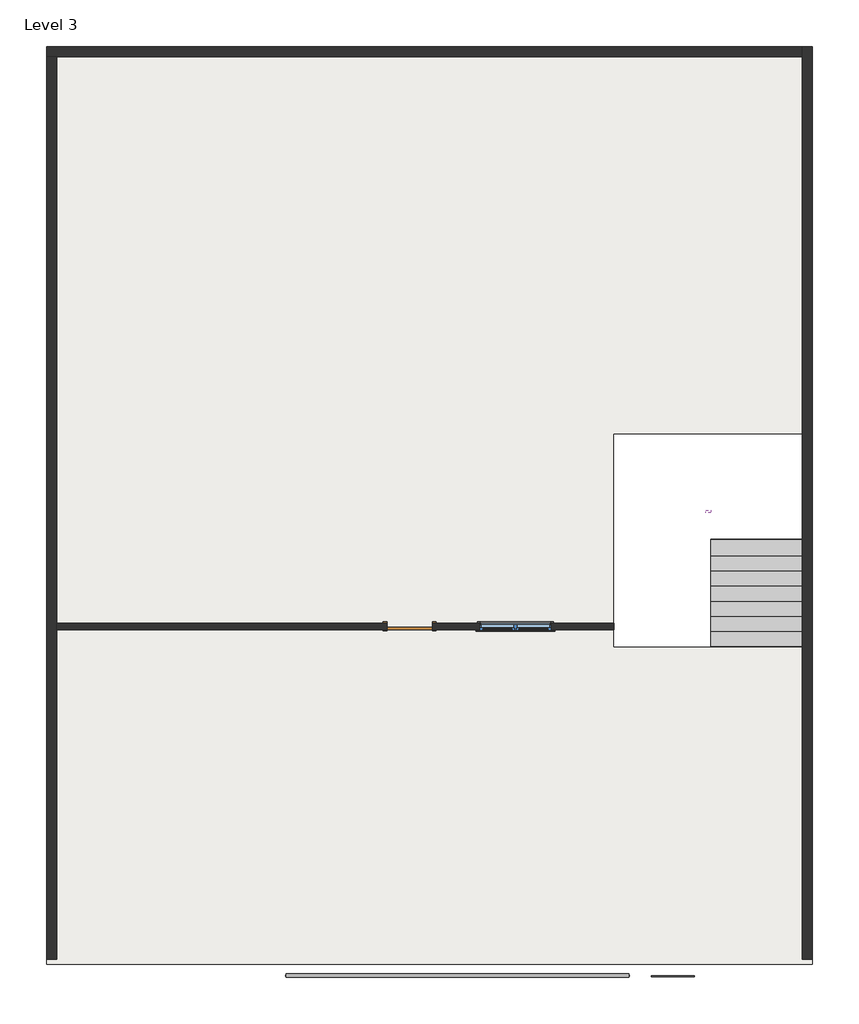
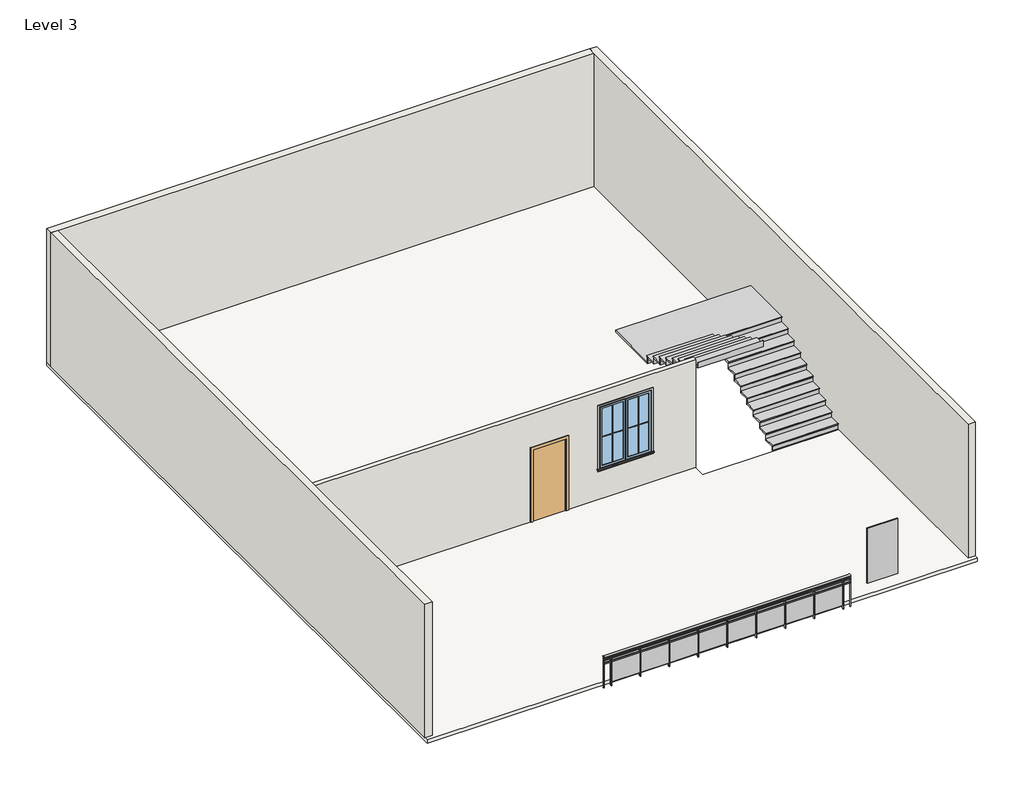
# One storey: 4 proxies, 4 walls, 1 door, 1 member, 1 plate, 1 railing, 1 slab, 1 stair flight, 1 window.
"""IFC4 building model written with IfcOpenShell, lengths in millimetres."""

from ifc_helpers import new_model, si_unit, point, frame, origin, place, context, project, spatial, polyline, ellipse_curve, trimmed, outline, extrude, faceted_brep, transform, mapped, element, save
from ifc_brep_helpers import plane_surface, extruded_surface, advanced_brep
from components import muntin_pattern_2x2_muntin_pattern_2x2_bff912c5, muntin_pattern_2x2_muntin_pattern_2x2_c2194282, trim_window_exterior_flat_with_sill_e04b3088, trim_window_interior_flat_picture_frame_2a7685fe, door_a1797ceb, system_panel_glazed_1c5a620b, stair_flight_059c6031, window_51a0d18f

model = new_model("IFC4")

# Units and contexts
model_context = context("Model", 3, world=origin())
ifc_project = project(units=[si_unit("LENGTHUNIT", "METRE", prefix="MILLI")], contexts=[model_context])

# Site, building, storey
site = spatial("IfcSite", under=ifc_project)
building = spatial("IfcBuilding", under=site)
storey = spatial("IfcBuildingStorey", under=building, Name="Level 3", Elevation=3962.4)

# Proxies
placement = place(None, origin())
muntin_pattern_2x2_muntin_pattern_2x2_shape = muntin_pattern_2x2_muntin_pattern_2x2_bff912c5(model_context)
element("IfcBuildingElementProxy", 1, Name="Muntin Pattern_2x2 : Muntin Pattern_2x2", ObjectType="Muntin Pattern_2x2 : Muntin Pattern_2x2", at=placement, inside=storey, context=model_context, shape_type="MappedRepresentation", body=[
    mapped(muntin_pattern_2x2_muntin_pattern_2x2_shape, transform((2360.2518946, -8297.1080955, 4946.65), x_axis=(-1.0, 0.0, 0.0), y_axis=(0.0, -1.0, 0.0), z_axis=(0.0, 0.0, 1.0))),
])
muntin_pattern_2x2_muntin_pattern_2x2_2_shape = muntin_pattern_2x2_muntin_pattern_2x2_c2194282(model_context)
element("IfcBuildingElementProxy", 2, Name="Muntin Pattern_2x2 : Muntin Pattern_2x2", ObjectType="Muntin Pattern_2x2 : Muntin Pattern_2x2", at=placement, inside=storey, context=model_context, shape_type="MappedRepresentation", body=[
    mapped(muntin_pattern_2x2_muntin_pattern_2x2_2_shape, transform((1639.5268946, -8297.1080955, 4946.65), x_axis=(1.0, 0.0, 0.0), y_axis=(0.0, 1.0, 0.0), z_axis=(0.0, 0.0, 1.0))),
])
trim_window_exterior_flat_with_sill_shape = trim_window_exterior_flat_with_sill_e04b3088(model_context)
element("IfcBuildingElementProxy", 3, Name="Trim-Window-Exterior-Flat : with Sill", ObjectType="Trim-Window-Exterior-Flat : with Sill", at=placement, inside=storey, context=model_context, shape_type="MappedRepresentation", body=[
    mapped(trim_window_exterior_flat_with_sill_shape, transform((1999.8893946, -8306.6330955, 6705.6), x_axis=(1.0, 0.0, 0.0), y_axis=(0.0, 0.0, 1.0), z_axis=(0.0, -1.0, 0.0))),
])
trim_window_interior_flat_picture_frame_shape = trim_window_interior_flat_picture_frame_2a7685fe(model_context)
element("IfcBuildingElementProxy", 4, Name="Trim-Window-Interior-Flat : Picture Frame", ObjectType="Trim-Window-Interior-Flat : Picture Frame", at=placement, inside=storey, context=model_context, shape_type="MappedRepresentation", body=[
    mapped(trim_window_interior_flat_picture_frame_shape, transform((1999.8893946, -8179.6330955, 6705.6), x_axis=(-1.0, 0.0, 0.0), y_axis=(0.0, 0.0, 1.0), z_axis=(0.0, 1.0, 0.0))),
])

# Door
door_shape = door_a1797ceb(model_context)
element("IfcDoor", 5, ObjectType="Single-Flush : 36\" x 84\"", at=placement, inside=storey, context=model_context, shape_type="MappedRepresentation", body=[
    mapped(door_shape, transform((-133.7106054, -8243.1330955, 3962.4), x_axis=(-1.0, 0.0, 0.0), y_axis=(0.0, -1.0, 0.0), z_axis=(0.0, 0.0, 1.0))),
])

# Member
element("IfcMember", 6, ObjectType="Stringer - 2\" Width", at=placement, inside=storey, context=model_context, shape_type="SweptSolid", body=[
    extrude(outline(polyline([(5940.6255016, -5904.9976656), (5940.6255016, -5955.7976656), (5839.0255016, -5955.7976656), (5839.0255016, -5904.9976656), (5940.6255016, -5904.9976656)])), frame((0.0, 0.0, 5418.2210526), z_axis=(0.0, 0.0, 1.0), x_axis=(1.0, 0.0, 0.0)), (0.0, 0.0, 1.0), 304.8),
])

# Plate
system_panel_glazed_shape = system_panel_glazed_1c5a620b(model_context)
element("IfcPlate", 7, ObjectType="System Panel : Glazed", at=placement, inside=storey, context=model_context, shape_type="MappedRepresentation", body=[
    mapped(system_panel_glazed_shape, transform((5174.2954883, -15325.4077095, 4495.8), x_axis=(1.0, 0.0, 0.0), y_axis=(0.0, 1.0, 0.0), z_axis=(0.0, 0.0, 1.0))),
])

# Railing
element("IfcRailing", 8, ObjectType="Glass Panel - Bottom Fill", at=placement, inside=storey, context=model_context, shape_type="SolidModel", body=[
    advanced_brep(
    [(-2628.7186876, -15240.8330955, 4876.8), (-2628.7186876, -15317.0330955, 4876.8), (4285.8893946, -15240.8330955, 4876.8), (4285.8893946, -15317.0330955, 4876.8)],
    [
        (0, 1, ellipse_curve(frame((-2628.7186876, -15278.9330955, 4876.8), z_axis=(-1.0, 0.0, 0.0), x_axis=(0.0, -1.0, 0.0)), 38.1, 28.575)),
        (1, 0, ellipse_curve(frame((-2628.7186876, -15278.9330955, 4876.8), z_axis=(-1.0, 0.0, 0.0), x_axis=(0.0, -1.0, 0.0)), 38.1, 28.575)),
        (2, 3, ellipse_curve(frame((4285.8893946, -15278.9330955, 4876.8), z_axis=(1.0, 0.0, 0.0), x_axis=(0.0, -1.0, 0.0)), 38.1, 28.575)),
        (3, 2, ellipse_curve(frame((4285.8893946, -15278.9330955, 4876.8), z_axis=(1.0, 0.0, 0.0), x_axis=(0.0, -1.0, 0.0)), 38.1, 28.575)),
        (0, 2),
        (3, 1),
    ],
    [
        plane_surface(frame((-2628.7186876, -15278.9330955, 4876.8), z_axis=(-1.0, 0.0, 0.0), x_axis=(0.0, 1.0, 0.0))),
        plane_surface(frame((4285.8893946, -15278.9330955, 4876.8), z_axis=(1.0, 0.0, 0.0), x_axis=(0.0, 1.0, 0.0))),
        extruded_surface(trimmed(ellipse_curve(frame((4285.8893946, -15278.9330955, 4876.8), z_axis=(-1.0, 0.0, 0.0), x_axis=(0.0, -1.0, 0.0)), 38.1, 28.575), [point((4285.8893946, -15240.8330955, 4876.8))], [point((4285.8893946, -15317.0330955, 4876.8))], True, "CARTESIAN"), (-6914.6080822, 0.0, 0.0), 6914.6080822),
        extruded_surface(trimmed(ellipse_curve(frame((4285.8893946, -15278.9330955, 4876.8), z_axis=(-1.0, 0.0, 0.0), x_axis=(0.0, -1.0, 0.0)), 38.1, 28.575), [point((4285.8893946, -15317.0330955, 4876.8))], [point((4285.8893946, -15240.8330955, 4876.8))], True, "CARTESIAN"), (-6914.6080822, 0.0, 0.0), 6914.6080822),
    ],
    [
        (0, [[1, 2]]),
        (1, [[3, 4]]),
        (2, [[-1, 5, -4, 6]]),
        (3, [[-2, -6, -3, -5]]),
    ],
),
    extrude(outline(polyline([(-2628.7186876, -15291.6330955), (-2628.7186876, -15266.2330955), (4285.8893946, -15266.2330955), (4285.8893946, -15291.6330955), (-2628.7186876, -15291.6330955)])), frame((0.0, 0.0, 4762.5), z_axis=(0.0, 0.0, 1.0), x_axis=(1.0, 0.0, 0.0)), (0.0, 0.0, 1.0), 25.4),
    extrude(outline(polyline([(-2628.7186876, -15291.6330955), (-2628.7186876, -15266.2330955), (4285.8893946, -15266.2330955), (4285.8893946, -15291.6330955), (-2628.7186876, -15291.6330955)])), frame((0.0, 0.0, 4660.9), z_axis=(0.0, 0.0, 1.0), x_axis=(1.0, 0.0, 0.0)), (0.0, 0.0, 1.0), 25.4),
    extrude(outline(polyline([(4073.4353535, -15304.3330955), (4073.4353535, -15253.5330955), (4086.1353535, -15253.5330955), (4086.1353535, -15304.3330955), (4073.4353535, -15304.3330955)])), frame((0.0, 0.0, 3962.4), z_axis=(0.0, 0.0, 1.0), x_axis=(1.0, 0.0, 0.0)), (0.0, 0.0, 1.0), 885.6788223),
    extrude(outline(polyline([(3266.9853535, -15272.3979385), (4079.7853535, -15272.3979385), (4079.7853535, -15278.7479385), (3266.9853535, -15278.7479385), (3266.9853535, -15272.3979385)])), frame((0.0, 0.0, 4064.0), z_axis=(0.0, 0.0, 1.0), x_axis=(1.0, 0.0, 0.0)), (0.0, 0.0, 1.0), 596.9),
    extrude(outline(polyline([(3260.6353535, -15304.3330955), (3260.6353535, -15253.5330955), (3273.3353535, -15253.5330955), (3273.3353535, -15304.3330955), (3260.6353535, -15304.3330955)])), frame((0.0, 0.0, 3962.4), z_axis=(0.0, 0.0, 1.0), x_axis=(1.0, 0.0, 0.0)), (0.0, 0.0, 1.0), 885.6788223),
    extrude(outline(polyline([(2454.1853535, -15272.3979385), (3266.9853535, -15272.3979385), (3266.9853535, -15278.7479385), (2454.1853535, -15278.7479385), (2454.1853535, -15272.3979385)])), frame((0.0, 0.0, 4064.0), z_axis=(0.0, 0.0, 1.0), x_axis=(1.0, 0.0, 0.0)), (0.0, 0.0, 1.0), 596.9),
    extrude(outline(polyline([(2447.8353535, -15304.3330955), (2447.8353535, -15253.5330955), (2460.5353535, -15253.5330955), (2460.5353535, -15304.3330955), (2447.8353535, -15304.3330955)])), frame((0.0, 0.0, 3962.4), z_axis=(0.0, 0.0, 1.0), x_axis=(1.0, 0.0, 0.0)), (0.0, 0.0, 1.0), 885.6788223),
    extrude(outline(polyline([(1641.3853535, -15272.3979385), (2454.1853535, -15272.3979385), (2454.1853535, -15278.7479385), (1641.3853535, -15278.7479385), (1641.3853535, -15272.3979385)])), frame((0.0, 0.0, 4064.0), z_axis=(0.0, 0.0, 1.0), x_axis=(1.0, 0.0, 0.0)), (0.0, 0.0, 1.0), 596.9),
    extrude(outline(polyline([(1635.0353535, -15304.3330955), (1635.0353535, -15253.5330955), (1647.7353535, -15253.5330955), (1647.7353535, -15304.3330955), (1635.0353535, -15304.3330955)])), frame((0.0, 0.0, 3962.4), z_axis=(0.0, 0.0, 1.0), x_axis=(1.0, 0.0, 0.0)), (0.0, 0.0, 1.0), 885.6788223),
    extrude(outline(polyline([(828.5853535, -15272.3979385), (1641.3853535, -15272.3979385), (1641.3853535, -15278.7479385), (828.5853535, -15278.7479385), (828.5853535, -15272.3979385)])), frame((0.0, 0.0, 4064.0), z_axis=(0.0, 0.0, 1.0), x_axis=(1.0, 0.0, 0.0)), (0.0, 0.0, 1.0), 596.9),
    extrude(outline(polyline([(822.2353535, -15304.3330955), (822.2353535, -15253.5330955), (834.9353535, -15253.5330955), (834.9353535, -15304.3330955), (822.2353535, -15304.3330955)])), frame((0.0, 0.0, 3962.4), z_axis=(0.0, 0.0, 1.0), x_axis=(1.0, 0.0, 0.0)), (0.0, 0.0, 1.0), 885.6788223),
    extrude(outline(polyline([(15.7853535, -15272.3979385), (828.5853535, -15272.3979385), (828.5853535, -15278.7479385), (15.7853535, -15278.7479385), (15.7853535, -15272.3979385)])), frame((0.0, 0.0, 4064.0), z_axis=(0.0, 0.0, 1.0), x_axis=(1.0, 0.0, 0.0)), (0.0, 0.0, 1.0), 596.9),
    extrude(outline(polyline([(9.4353535, -15304.3330955), (9.4353535, -15253.5330955), (22.1353535, -15253.5330955), (22.1353535, -15304.3330955), (9.4353535, -15304.3330955)])), frame((0.0, 0.0, 3962.4), z_axis=(0.0, 0.0, 1.0), x_axis=(1.0, 0.0, 0.0)), (0.0, 0.0, 1.0), 885.6788223),
    extrude(outline(polyline([(-797.0146465, -15272.3979385), (15.7853535, -15272.3979385), (15.7853535, -15278.7479385), (-797.0146465, -15278.7479385), (-797.0146465, -15272.3979385)])), frame((0.0, 0.0, 4064.0), z_axis=(0.0, 0.0, 1.0), x_axis=(1.0, 0.0, 0.0)), (0.0, 0.0, 1.0), 596.9),
    extrude(outline(polyline([(-803.3646465, -15304.3330955), (-803.3646465, -15253.5330955), (-790.6646465, -15253.5330955), (-790.6646465, -15304.3330955), (-803.3646465, -15304.3330955)])), frame((0.0, 0.0, 3962.4), z_axis=(0.0, 0.0, 1.0), x_axis=(1.0, 0.0, 0.0)), (0.0, 0.0, 1.0), 885.6788223),
    extrude(outline(polyline([(-1609.8146465, -15272.3979385), (-797.0146465, -15272.3979385), (-797.0146465, -15278.7479385), (-1609.8146465, -15278.7479385), (-1609.8146465, -15272.3979385)])), frame((0.0, 0.0, 4064.0), z_axis=(0.0, 0.0, 1.0), x_axis=(1.0, 0.0, 0.0)), (0.0, 0.0, 1.0), 596.9),
    extrude(outline(polyline([(-1616.1646465, -15304.3330955), (-1616.1646465, -15253.5330955), (-1603.4646465, -15253.5330955), (-1603.4646465, -15304.3330955), (-1616.1646465, -15304.3330955)])), frame((0.0, 0.0, 3962.4), z_axis=(0.0, 0.0, 1.0), x_axis=(1.0, 0.0, 0.0)), (0.0, 0.0, 1.0), 885.6788223),
    extrude(outline(polyline([(-2422.6146465, -15272.3979385), (-1609.8146465, -15272.3979385), (-1609.8146465, -15278.7479385), (-2422.6146465, -15278.7479385), (-2422.6146465, -15272.3979385)])), frame((0.0, 0.0, 4064.0), z_axis=(0.0, 0.0, 1.0), x_axis=(1.0, 0.0, 0.0)), (0.0, 0.0, 1.0), 596.9),
    extrude(outline(polyline([(-2428.9646465, -15304.3330955), (-2428.9646465, -15253.5330955), (-2416.2646465, -15253.5330955), (-2416.2646465, -15304.3330955), (-2428.9646465, -15304.3330955)])), frame((0.0, 0.0, 3962.4), z_axis=(0.0, 0.0, 1.0), x_axis=(1.0, 0.0, 0.0)), (0.0, 0.0, 1.0), 885.6788223),
    extrude(outline(polyline([(4273.1893946, -15288.4580955), (4273.1893946, -15269.4080955), (4292.2393946, -15269.4080955), (4292.2393946, -15288.4580955), (4273.1893946, -15288.4580955)])), frame((0.0, 0.0, 3962.4), z_axis=(0.0, 0.0, 1.0), x_axis=(1.0, 0.0, 0.0)), (0.0, 0.0, 1.0), 885.6788223),
    extrude(outline(polyline([(-2635.0686876, -15288.4580955), (-2635.0686876, -15269.4080955), (-2616.0186876, -15269.4080955), (-2616.0186876, -15288.4580955), (-2635.0686876, -15288.4580955)])), frame((0.0, 0.0, 3962.4), z_axis=(0.0, 0.0, 1.0), x_axis=(1.0, 0.0, 0.0)), (0.0, 0.0, 1.0), 885.6788223),
])

# Slab
element("IfcSlab", 9, ObjectType="Generic - 4\"", at=placement, inside=storey, context=model_context, shape_type="SweptSolid", body=[
    extrude(outline(polyline([(-7454.7186876, -15050.3330955), (-7454.7186876, 3440.8669045), (7988.4813124, 3440.8669045), (7988.4813124, -15050.3330955), (-7454.7186876, -15050.3330955)]), holes=[polyline([(7797.9813124, -4367.7173694), (3981.0893946, -4367.7173694), (3981.0893946, -8648.1976656), (7797.9813124, -8648.1976656), (7797.9813124, -4367.7173694)])]), frame((0.0, 0.0, 3860.8), z_axis=(0.0, 0.0, 1.0), x_axis=(1.0, 0.0, 0.0)), (0.0, 0.0, 1.0), 101.6),
])

# Stair flight
stair_flight_shape = stair_flight_059c6031(model_context)
element("IfcStairFlight", 10, ObjectType="2\" Tread 1\" Nosing 1/4\" Riser", at=placement, inside=storey, context=model_context, shape_type="MappedRepresentation", body=[
    mapped(stair_flight_shape, transform((0.0, 0.0, 0.0), x_axis=(1.0, 0.0, 0.0), y_axis=(0.0, 1.0, 0.0), z_axis=(0.0, 0.0, 1.0))),
])

# Walls
element("IfcWall", 11, ObjectType="Generic - 5\"", at=placement, inside=storey, context=model_context, shape_type="SweptSolid", body=[
    extrude(outline(polyline([(3962.4, -7251.5186876), (3962.4, -590.9106054), (6096.0, -590.9106054), (6096.0, 323.4893946), (3962.4, 323.4893946), (3962.4, 3981.0893946), (7162.8, 3981.0893946), (7162.8, -7251.5186876), (3962.4, -7251.5186876)]), holes=[polyline([(6705.6, 1275.9893946), (6705.6, 2723.7893946), (4876.8, 2723.7893946), (4876.8, 1275.9893946), (6705.6, 1275.9893946)])]), frame((0.0, -8306.6330955, 0.0), z_axis=(0.0, 1.0, 0.0), x_axis=(0.0, 0.0, 1.0)), (0.0, 0.0, 1.0), 127.0),
])
element("IfcWall", 12, ObjectType="Generic - 8\"", at=placement, inside=storey, context=model_context, shape_type="Brep", body=[
    faceted_brep([(7988.4813124, -14948.7330955, 3962.4), (7988.4813124, 3440.8669045, 3962.4), (7988.4813124, 3440.8669045, 7924.8), (7988.4813124, -14948.7330955, 7924.8), (7785.2813124, -14948.7330955, 3962.4), (7785.2813124, -14948.7330955, 7924.8), (7785.2813124, 3237.6669045, 7924.8), (7785.2813124, 3440.8669045, 7924.8), (7785.2813124, 3440.8669045, 3962.4), (7785.2813124, 3237.6669045, 3962.4)], [[[0, 1, 2, 3]], [[4, 5, 6, 7, 8, 9]], [[1, 0, 4, 9, 8]], [[3, 2, 7, 6, 5]], [[0, 3, 5, 4]], [[2, 1, 8, 7]]]),
])
element("IfcWall", 13, ObjectType="Generic - 8\"", at=placement, inside=storey, context=model_context, shape_type="Brep", body=[
    faceted_brep([(7785.2813124, 3440.8669045, 3962.4), (-7454.7186876, 3440.8669045, 3962.4), (-7454.7186876, 3440.8669045, 7924.8), (7785.2813124, 3440.8669045, 7924.8), (7785.2813124, 3237.6669045, 3962.4), (7785.2813124, 3237.6669045, 7924.8), (-7251.5186876, 3237.6669045, 7924.8), (-7454.7186876, 3237.6669045, 7924.8), (-7454.7186876, 3237.6669045, 3962.4), (-7251.5186876, 3237.6669045, 3962.4)], [[[0, 1, 2, 3]], [[4, 5, 6, 7, 8, 9]], [[1, 0, 4, 9, 8]], [[3, 2, 7, 6, 5]], [[0, 3, 5, 4]], [[2, 1, 8, 7]]]),
])
element("IfcWall", 14, ObjectType="Generic - 8\"", at=placement, inside=storey, context=model_context, shape_type="Brep", body=[
    faceted_brep([(-7454.7186876, 3237.6669045, 3962.4), (-7454.7186876, -14948.7330955, 3962.4), (-7454.7186876, -14948.7330955, 7924.8), (-7454.7186876, 3237.6669045, 7924.8), (-7251.5186876, 3237.6669045, 3962.4), (-7251.5186876, 3237.6669045, 7924.8), (-7251.5186876, -14948.7330955, 7924.8), (-7251.5186876, -14948.7330955, 3962.4), (-7251.5186876, -8306.6330955, 3962.4), (-7251.5186876, -8179.6330955, 3962.4)], [[[0, 1, 2, 3]], [[4, 5, 6, 7, 8, 9]], [[1, 0, 4, 9, 8, 7]], [[2, 1, 7, 6]], [[3, 2, 6, 5]], [[0, 3, 5, 4]]]),
])

# Window
window_shape = window_51a0d18f(model_context)
element("IfcWindow", 15, ObjectType="Window-Casement-Double : 57\" x 72\"", at=placement, inside=storey, context=model_context, shape_type="MappedRepresentation", body=[
    mapped(window_shape, transform((1999.8893946, -8243.1330955, 3962.4), x_axis=(-1.0, 0.0, 0.0), y_axis=(0.0, -1.0, 0.0), z_axis=(0.0, 0.0, 1.0))),
])

save(model, "model.ifc")

# Revit data of these elements
# Type "Muntin Pattern_2x2 : Muntin Pattern_2x2"
#   Width [instance default] = 4' - 0"
#   Thickness = 0' - 0 1/2"
#   Height [instance default] = 4' - 0"
#   Distance = 0' - 0 3/4"
#   Interior Material [instance default] = none
#   Exterior Material [instance default] = none
#   Default Elevation = 0
# Type "Trim-Window-Exterior-Flat : with Sill"
#   Trim Width = 0' - 2 1/4"
#   Trim Thickness_Picture Frame = 0' - 1 1/4"
#   Trim Thickness_with Sill = 0' - 0 3/4"
#   Sill Thickness = 0' - 1 1/4"
#   Opening Width [instance default] = 2' - 0"
#   Opening Height [instance default] = 3' - 0"
#   Default Elevation = 4' - 0"
#   Sill = yes
#   Picture Frame = no
#   Trim Material [instance default] = none
# Type "Trim-Window-Interior-Flat : Picture Frame"
#   Trim Thickness_Picture Frame = 0' - 1 1/4"
#   Trim Width = 0' - 2 1/4"
#   Trim Thickness_with Sill = 0' - 0 3/4"
#   Sill Thickness = 0' - 1 1/4"
#   Opening Width [instance default] = 2' - 0"
#   Opening Height [instance default] = 3' - 0"
#   Default Elevation = 4' - 0"
#   Sill = no
#   Picture Frame = yes
#   Trim Material [instance default] = none
# Type "Single-Flush : 36\" x 84\""
#   Type Mark = "1"
#   Construction Type Id = "MDOOR"
#   Assembly Code = "C1020"
#   Analytic Construction = "Metal"
#   Thickness = 0' - 2"
#   Heat Transfer Coefficient (U) = 0.651978 BTU/(h·ft²·°F)
#   Height = 7' - 0"
#   Trim Projection Ext = 0' - 1"
#   Trim Projection Int = 0' - 1"
#   Trim Width = 0' - 3"
#   Width = 3' - 0"
#   Define Thermal Properties by = 1
#   Define Thermal Properties by = 1
#   Door Material = Door - Panel
#   Frame Material = Door - Frame
#   Visual Light Transmittance = 0
#   Solar Heat Gain Coefficient = 0
#   Function = (empty or 0)
#   Wall Closure = (empty or 0)
# Type "System Panel : Glazed"
#   Construction Type Id = "GSP4R"
#   Analytic Construction = "1/8 in Pilkington single glazing"
#   Visual Light Transmittance = 0.9
#   Solar Heat Gain Coefficient = 0.86
#   Heat Transfer Coefficient (U) = 1.18115 BTU/(h·ft²·°F)
#   Define Thermal Properties by = 1
# Type "Glass Panel - Bottom Fill"
#   Assembly Code = "C2010400"
#   built-in parameter 1008612 = 0.0416667 (stored number, unit not read)
#   built-in parameter 1008611 = 0.0416667 (stored number, unit not read)
#   built-in parameter 1008609 = 0.333333 (stored number, unit not read)
#   built-in parameter 1008604 = 0.166667 (stored number, unit not read)
#   built-in parameter 1008603 = 0.166667 (stored number, unit not read)
#   Railing Height = 3' - 0"
#   built-in parameter 1008630 = 2
#   built-in parameter 1008610 = 2
#   built-in parameter 1008618 = Baluster - Square : 3/4"
# Type "Generic - 4\""
#   Assembly Code = "B1010"
#   Function = 0
#   Layers, outside or top first: 0' - 4" no material (function 1)
# Type "Generic - 5\""
#   Assembly Code = "B2010"
#   Layers, outside or top first: 0' - 5" no material (function 1)
# Type "Generic - 8\""
#   Assembly Code = "B2010"
#   Layers, outside or top first: 0' - 8" no material (function 1)
# Type "Window-Casement-Double : 57\" x 72\""
#   Type Mark = "17"
#   Fire Rating = "0.5h"
#   Assembly Code = "B2020100"
#   Analytic Construction = "Double glazing - domestic"
#   Frame Extension [instance default] = 0' - 0 1/4"
#   Window Inset [instance default] = 0' - 0"
#   Wall Thickness [instance default] = 0' - 6"
#   Interior Wall Closure [instance default] = 0' - 2 1/4"
#   Half Width = 2' - 4 1/2"
#   Visual Light Transmittance = 0.81
#   Thermal Resistance (R) = 1.8146 (h·ft²·°F)/BTU
#   Solar Heat Gain Coefficient = 0.76
#   Rough Width = 4' - 9 1/2"
#   Rough Height = 6' - 0 1/2"
#   Height = 6' - 0"
#   Heat Transfer Coefficient (U) = 0.5511 BTU/(h·ft²·°F)
#   Exterior Wall Closure [instance default] = 0' - 1 1/4"
#   Extension Jamb [instance default] = 0' - 2 1/4"
#   Default Sill Height = 3' - 0"
#   Width = 4' - 9"
#   Define Thermal Properties by = 0
#   Muntin Visibility = yes
#   Interior Trim Visibility [instance default] = yes
#   Exterior Trim Visibility [instance default] = yes
#   Extension Jamb Visibility [instance default] = yes
#   Interior Trim Material = Wood - Stained
#   Muntin Pattern = Muntin Pattern_2x2 : Muntin Pattern_2x2
#   Interior Trim = Trim-Window-Interior-Flat : Picture Frame
#   Interior Frame Material = Wood - Stained
#   Glass Panel Material = Glass
#   Exterior Trim Material = Clad - White
#   Exterior Trim = Trim-Window-Exterior-Flat : with Sill
#   Exterior Frame Material = Clad - White
#   Wall Closure = (empty or 0)
# Elements 1, 2 (IfcBuildingElementProxy, "Muntin Pattern_2x2 : Muntin Pattern_2x2")
#   Width = 1' - 11 1/8"
#   Height = 5' - 6 1/2"
#   Interior Material = Wood - Stained
#   Exterior Material = Clad - White
#   Phase Created = New Construction
#   Materials on its faces: "Clad - White", "Wood - Stained"
# Element 3 (IfcBuildingElementProxy, "Trim-Window-Exterior-Flat : with Sill")
#   Opening Width = 4' - 9"
#   Opening Height = 6' - 0"
#   Trim Material = Clad - White
#   Phase Created = New Construction
#   Materials on its faces: "Clad - White"
# Element 4 (IfcBuildingElementProxy, "Trim-Window-Interior-Flat : Picture Frame")
#   Opening Width = 4' - 9"
#   Opening Height = 6' - 0"
#   Trim Material = Wood - Stained
#   Phase Created = New Construction
#   Materials on its faces: "Wood - Stained"
# Element 5 (IfcDoor, "Single-Flush : 36\" x 84\"")
#   Phase Created = New Construction
#   Materials on its faces: "Door - Frame", "Door - Panel"
# Element 6 (IfcMember, "Stringer - 2\" Width")
#   Phase Created = New Construction
# Element 7 (IfcPlate, "System Panel : Glazed")
#   Phase Created = New Construction
#   Materials on its faces: "Glass"
# Element 8 (IfcRailing, "Glass Panel - Bottom Fill")
#   Phase Created = New Construction
#   Materials on its faces: "Glass"
# Element 9 (IfcSlab, "Generic - 4\"")
#   built-in parameter 1001955 = -1.5708 (stored number, unit not read)
#   Height Offset From Level = 0' - 0"
#   Phase Created = New Construction
#   Materials on its faces: "Default Floor", "floor"
# Element 10 (IfcStairFlight, "2\" Tread 1\" Nosing 1/4\" Riser")
#   Phase Created = New Construction
# Element 11 (IfcWall, "Generic - 5\"")
#   Top Offset = 0' - 0"
#   Base Offset = 0' - 0"
#   wall height = 10' - 6"
#   Phase Created = New Construction
#   Base Constraint = Level 3
#   Top Constraint = Level 4
#   Materials on its faces: "Default Wall"
# Elements 12, 13, 14 (IfcWall, "Generic - 8\"")
#   Top Offset = 13' - 0"
#   Base Offset = 0' - 0"
#   wall height = 13' - 0"
#   Phase Created = New Construction
#   Base Constraint = Level 3
#   Top Constraint = Level 3
#   Materials on its faces: "Default Wall", "Clad - White"
# Element 15 (IfcWindow, "Window-Casement-Double : 57\" x 72\"")
#   Mark = "2"
#   Window Inset = 0' - 0"
#   Interior Wall Closure = 0' - 2 1/4"
#   Frame Extension = 0' - 0 1/4"
#   Exterior Wall Closure = 0' - 1 1/4"
#   Interior Trim Visibility = yes
#   Exterior Trim Visibility = yes
#   Phase Created = New Construction
#   Materials on its faces: "Wood - Stained", "Glass", "Clad - White"
# Materials
#   "Door - Panel": class "Wood", colour RGB 210 159 95, transparency 0, Cost = 0
#   "Door - Frame": colour RGB 118 70 51, transparency 0, Cost = 0
#   "Wood - Stained": class "Wood", colour RGB 224 178 126, transparency 0, Cost = 0
#   "Glass": class "Glass", colour RGB 0 128 192, transparency 0.75, Description = "Soda Lime Glass", Cost = 0
#   "Clad - White": class "Wood", colour RGB 242 242 238, transparency 0, Cost = 0
#   "Default Floor": colour RGB 128 128 128, transparency 0, Cost = 0
#   "floor": class "Generic", colour RGB 255 207 159, transparency 0, Cost = 0
#   "Default Wall": colour RGB 128 128 128, transparency 0, Cost = 0
